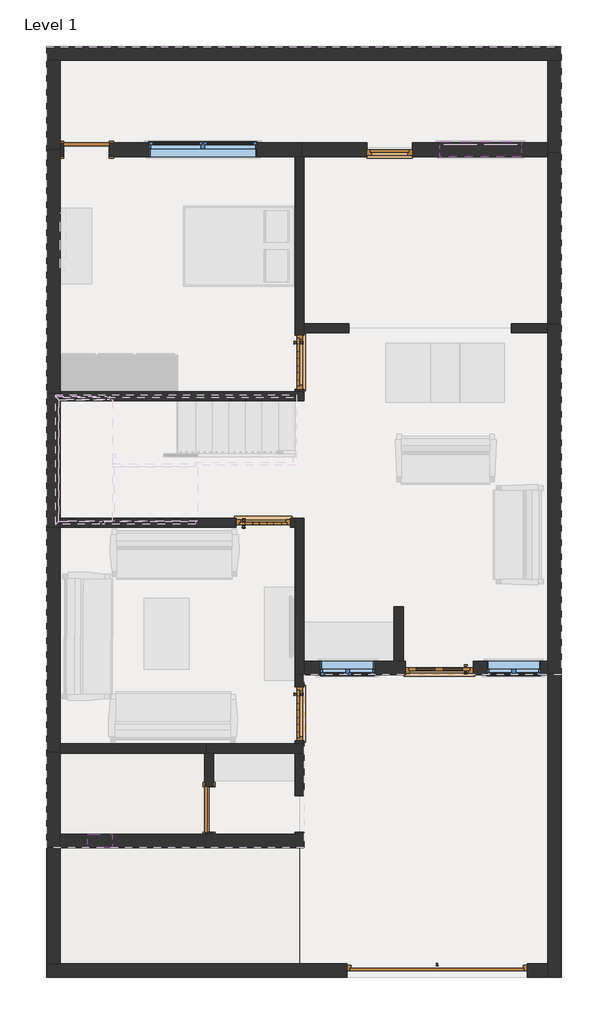
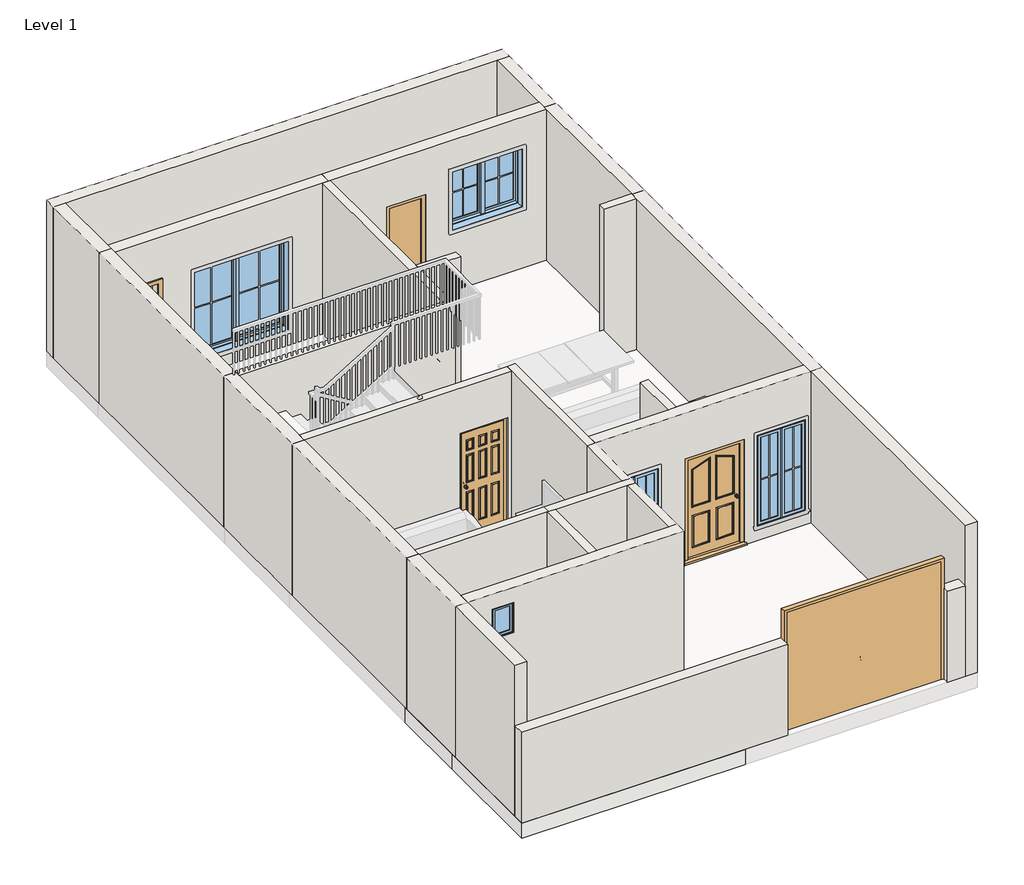
# One storey, part 1 of 3: 28 walls, 8 doors, 5 windows, 2 slabs.
"""IFC4 building model written with IfcOpenShell, lengths in millimetres."""

from ifc_helpers import new_model, si_unit, point, frame, frame_2d, origin, origin_with_axes, place, context, project, spatial, polyline, circle_curve, trimmed, segment, composite_curve, outline, extrude, faceted_brep, transform, mapped, element, save
from components import doors_concept_extsgl_762x2134mm_2_ed5749d6, doors_extsgl_12_1143x2134mm_2_6d3613a0, doors_extsgl_3_914x2134mm_2_3fd9b232, doors_garage_horz_pnl_3048x2438mm_2_abfe55f9, door_e2b13fe9, door_5e1232af, window_aa618e30, window_5590b26e, window_ecc443c5, window_ce442eab

model = new_model("IFC4")

# Units and contexts
model_context = context("Model", 3, world=origin())
ifc_project = project(units=[si_unit("LENGTHUNIT", "METRE", prefix="MILLI")], contexts=[model_context])

# Site, building, storey
site = spatial("IfcSite", under=ifc_project)
building = spatial("IfcBuilding", under=site)
storey = spatial("IfcBuildingStorey", under=building, Name="Level 1", Elevation=0.0)

# Doors
placement = place(None, origin())
doors_concept_extsgl_762x2134mm_2_shape = doors_concept_extsgl_762x2134mm_2_ed5749d6(model_context)
element("IfcDoor", 1, ObjectType="Doors_Concept_ExtSgl : 762x2134mm 2", at=placement, inside=storey, context=model_context, shape_type="MappedRepresentation", body=[
    mapped(doors_concept_extsgl_762x2134mm_2_shape, transform((214.6994028, 7031.3870892, 0.0), x_axis=(-1.0, 0.0, 0.0), y_axis=(0.0, -1.0, 0.0), z_axis=(0.0, 0.0, 1.0))),
])
doors_extsgl_12_1143x2134mm_2_shape = doors_extsgl_12_1143x2134mm_2_6d3613a0(model_context)
element("IfcDoor", 2, ObjectType="Doors_ExtSgl_12 : 1143x2134mm 2", at=placement, inside=storey, context=model_context, shape_type="MappedRepresentation", body=[
    mapped(doors_extsgl_12_1143x2134mm_2_shape, transform((1052.8994028, -1706.2129108, 0.0), x_axis=(-1.0, 0.0, 0.0), y_axis=(0.0, -1.0, 0.0), z_axis=(0.0, 0.0, 1.0))),
])
doors_extsgl_3_914x2134mm_2_shape = doors_extsgl_3_914x2134mm_2_3fd9b232(model_context)
element("IfcDoor", 3, ObjectType="Doors_ExtSgl_3 : 914x2134mm 2", at=placement, inside=storey, context=model_context, shape_type="MappedRepresentation", body=[
    mapped(doors_extsgl_3_914x2134mm_2_shape, transform((-1918.9339305, 744.8870892, 0.0), x_axis=(1.0, 0.0, 0.0), y_axis=(0.0, 1.0, 0.0), z_axis=(0.0, 0.0, 1.0))),
])
element("IfcDoor", 4, ObjectType="Doors_ExtSgl_3 : 914x2134mm 2", at=placement, inside=storey, context=model_context, shape_type="MappedRepresentation", body=[
    mapped(doors_extsgl_3_914x2134mm_2_shape, transform((-1309.3005972, -2480.8795775, 0.0), x_axis=(0.0, -1.0, 0.0), y_axis=(1.0, 0.0, 0.0), z_axis=(0.0, 0.0, 1.0))),
])
element("IfcDoor", 5, ObjectType="Doors_ExtSgl_3 : 914x2134mm 2", at=placement, inside=storey, context=model_context, shape_type="MappedRepresentation", body=[
    mapped(doors_extsgl_3_914x2134mm_2_shape, transform((-1309.3005972, 3450.0204225, 0.0), x_axis=(0.0, -1.0, 0.0), y_axis=(1.0, 0.0, 0.0), z_axis=(0.0, 0.0, 1.0))),
])
doors_garage_horz_pnl_3048x2438mm_2_shape = doors_garage_horz_pnl_3048x2438mm_2_abfe55f9(model_context)
element("IfcDoor", 6, ObjectType="Doors_Garage_Horz_Pnl : 3048x2438mm 2", at=placement, inside=storey, context=model_context, shape_type="MappedRepresentation", body=[
    mapped(doors_garage_horz_pnl_3048x2438mm_2_shape, transform((626.2994028, -6811.6129108, 0.0), x_axis=(1.0, 0.0, 0.0), y_axis=(0.0, 1.0, 0.0), z_axis=(0.0, 0.0, 1.0))),
])
door_shape = door_e2b13fe9(model_context)
element("IfcDoor", 7, ObjectType="Single-Flush : 30\" x 80\" 2", at=placement, inside=storey, context=model_context, shape_type="MappedRepresentation", body=[
    mapped(door_shape, transform((-2833.3005972, -4093.8129108, 0.0), x_axis=(0.0, -1.0, 0.0), y_axis=(1.0, 0.0, 0.0), z_axis=(0.0, 0.0, 1.0))),
])
door_2_shape = door_5e1232af(model_context)
element("IfcDoor", 8, ObjectType="Single-Flush : 30\" x 80\" 2", at=placement, inside=storey, context=model_context, shape_type="MappedRepresentation", body=[
    mapped(door_2_shape, transform((-4903.4005972, 7031.3870892, 0.0), x_axis=(-1.0, 0.0, 0.0), y_axis=(0.0, -1.0, 0.0), z_axis=(0.0, 0.0, 1.0))),
])

# Slabs
element("IfcSlab", 9, ObjectType="Generic - 12\"", at=placement, inside=storey, context=model_context, shape_type="SweptSolid", body=[
    extrude(outline(polyline([(-2833.3005972, -3065.1129108), (-2833.3005972, -4627.2129108), (-5576.5005972, -4627.2129108), (-5576.5005972, -3065.1129108), (-2833.3005972, -3065.1129108)])), frame((0.0, 0.0, -304.8), z_axis=(0.0, 0.0, 1.0), x_axis=(1.0, 0.0, 0.0)), (0.0, 0.0, 1.0), 304.8),
])
element("IfcSlab", 10, ObjectType="Generic - 12\"", at=placement, inside=storey, context=model_context, shape_type="SweptSolid", body=[
    extrude(outline(polyline([(-1309.3005972, -4627.2129108), (-1309.3005972, -6925.9129108), (-5576.5005972, -6925.9129108), (-5576.5005972, -4627.2129108), (-1309.3005972, -4627.2129108)])), frame((0.0, 0.0, -304.8), z_axis=(0.0, 0.0, 1.0), x_axis=(1.0, 0.0, 0.0)), (0.0, 0.0, 1.0), 304.8),
])

# Walls
element("IfcWall", 11, ObjectType="Generic - 8\" 9\"", at=placement, inside=storey, context=model_context, shape_type="Brep", body=[
    faceted_brep([(-5576.5005972, 8542.6870892, 0.0), (-5347.9005972, 8542.6870892, 0.0), (2881.6994028, 8542.6870892, 0.0), (3110.2994028, 8542.6870892, 0.0), (3110.2994028, 8542.6870892, 3048.0), (2881.6994028, 8542.6870892, 3048.0), (-5347.9005972, 8542.6870892, 3048.0), (-5576.5005972, 8542.6870892, 3048.0), (-5576.5005972, 8771.2870892, 0.0), (-5576.5005972, 8771.2870892, 3048.0), (3110.2994028, 8771.2870892, 3048.0), (3110.2994028, 8771.2870892, 0.0)], [[[0, 1, 2, 3, 4, 5, 6, 7]], [[8, 9, 10, 11]], [[3, 2, 1, 0, 8, 11]], [[7, 6, 5, 4, 10, 9]], [[4, 3, 11, 10]], [[0, 7, 9, 8]]]),
])
element("IfcWall", 12, ObjectType="Generic - 8\" 9\"", at=placement, inside=storey, context=model_context, shape_type="Brep", body=[
    faceted_brep([(2881.6994028, 8542.6870892, 0.0), (2881.6994028, 7145.6870892, 0.0), (2881.6994028, 6980.5870892, 0.0), (2881.6994028, 6980.5870892, 3048.0), (2881.6994028, 7145.6870892, 3048.0), (2881.6994028, 8542.6870892, 3048.0), (3110.2994028, 8542.6870892, 0.0), (3110.2994028, 8542.6870892, 3048.0), (3110.2994028, 6980.5870892, 3048.0), (3110.2994028, 6980.5870892, 0.0)], [[[0, 1, 2, 3, 4, 5]], [[6, 7, 8, 9]], [[2, 1, 0, 6, 9]], [[3, 2, 9, 8]], [[5, 4, 3, 8, 7]], [[0, 5, 7, 6]]]),
])
element("IfcWall", 13, ObjectType="Generic - 8\" 9\"", at=placement, inside=storey, context=model_context, shape_type="Brep", body=[
    faceted_brep([(2881.6994028, -6697.3129108, 1828.8), (2881.6994028, -6697.3129108, 0.0), (2538.7994028, -6697.3129108, 0.0), (2538.7994028, -6697.3129108, 1828.8), (2881.6994028, -6925.9129108, 0.0), (2881.6994028, -6925.9129108, 1828.8), (2538.7994028, -6925.9129108, 1828.8), (2538.7994028, -6925.9129108, 0.0)], [[[0, 1, 2, 3]], [[4, 5, 6, 7]], [[1, 4, 7, 2]], [[5, 0, 3, 6]], [[1, 0, 5, 4]], [[3, 2, 7, 6]]]),
    faceted_brep([(-5576.5005972, -6697.3129108, 0.0), (-5576.5005972, -6697.3129108, 1828.8), (-509.2005972, -6697.3129108, 1828.8), (-509.2005972, -6697.3129108, 0.0), (-5347.9005972, -6697.3129108, 0.0), (-5576.5005972, -6925.9129108, 1828.8), (-5576.5005972, -6925.9129108, 0.0), (-509.2005972, -6925.9129108, 0.0), (-509.2005972, -6925.9129108, 1828.8)], [[[0, 1, 2, 3, 4]], [[5, 6, 7, 8]], [[6, 0, 4, 3, 7]], [[1, 5, 8, 2]], [[1, 0, 6, 5]], [[3, 2, 8, 7]]]),
])
element("IfcWall", 14, ObjectType="Generic - 8\" 9\"", at=placement, inside=storey, context=model_context, shape_type="Brep", body=[
    faceted_brep([(-5576.5005972, 8542.6870892, 0.0), (-5576.5005972, 7031.3870892, 0.0), (-5576.5005972, 7031.3870892, 3048.0), (-5576.5005972, 8542.6870892, 3048.0), (-5347.9005972, 8542.6870892, 0.0), (-5347.9005972, 8542.6870892, 3048.0), (-5347.9005972, 7145.6870892, 3048.0), (-5347.9005972, 7031.3870892, 3048.0), (-5347.9005972, 7031.3870892, 0.0), (-5347.9005972, 7145.6870892, 0.0)], [[[0, 1, 2, 3]], [[4, 5, 6, 7, 8, 9]], [[1, 0, 4, 9, 8]], [[2, 1, 8, 7]], [[3, 2, 7, 6, 5]], [[0, 3, 5, 4]]]),
])
element("IfcWall", 15, ObjectType="Generic - 8\" 9\"", at=placement, inside=storey, context=model_context, shape_type="Brep", body=[
    faceted_brep([(-5347.9005972, -4741.5129108, 0.0), (-1233.1005972, -4741.5129108, 0.0), (-1233.1005972, -4741.5129108, 3048.0), (-5347.9005972, -4741.5129108, 3048.0), (-4878.0005972, -4741.5129108, 2743.2), (-4471.6005972, -4741.5129108, 2743.2), (-4471.6005972, -4741.5129108, 2133.6), (-4878.0005972, -4741.5129108, 2133.6), (-5347.9005972, -4512.9129108, 0.0), (-5347.9005972, -4512.9129108, 3048.0), (-2909.5005972, -4512.9129108, 3048.0), (-2757.1005972, -4512.9129108, 3048.0), (-1385.5005972, -4512.9129108, 3048.0), (-1233.1005972, -4512.9129108, 3048.0), (-1233.1005972, -4512.9129108, 0.0), (-1385.5005972, -4512.9129108, 0.0), (-2757.1005972, -4512.9129108, 0.0), (-2909.5005972, -4512.9129108, 0.0), (-4878.0005972, -4512.9129108, 2743.2), (-4878.0005972, -4512.9129108, 2133.6), (-4471.6005972, -4512.9129108, 2133.6), (-4471.6005972, -4512.9129108, 2743.2)], [[[0, 1, 2, 3], [4, 5, 6, 7]], [[8, 9, 10, 11, 12, 13, 14, 15, 16, 17], [18, 19, 20, 21]], [[1, 0, 8, 17, 16, 15, 14]], [[3, 2, 13, 12, 11, 10, 9]], [[0, 3, 9, 8]], [[2, 1, 14, 13]], [[19, 18, 4, 7]], [[20, 19, 7, 6]], [[21, 20, 6, 5]], [[18, 21, 5, 4]]]),
])
element("IfcWall", 16, ObjectType="Generic - 8\" 9\"", at=placement, inside=storey, context=model_context, shape_type="Brep", body=[
    faceted_brep([(481.3994028, -1591.9129108, 2133.6), (481.3994028, -1591.9129108, 0.0), (443.2994028, -1591.9129108, 0.0), (290.8994028, -1591.9129108, 0.0), (-1233.1005972, -1591.9129108, 0.0), (-1233.1005972, -1591.9129108, 3048.0), (290.8994028, -1591.9129108, 3048.0), (443.2994028, -1591.9129108, 3048.0), (2881.6994028, -1591.9129108, 3048.0), (2881.6994028, -1591.9129108, 0.0), (1624.3994028, -1591.9129108, 0.0), (1624.3994028, -1591.9129108, 2133.6), (-953.7005972, -1591.9129108, 2133.6), (-953.7005972, -1591.9129108, 304.8), (-39.3005972, -1591.9129108, 304.8), (-39.3005972, -1591.9129108, 2133.6), (1852.9994028, -1591.9129108, 2133.6), (1852.9994028, -1591.9129108, 304.8), (2767.3994028, -1591.9129108, 304.8), (2767.3994028, -1591.9129108, 2133.6), (-1233.1005972, -1820.5129108, 0.0), (481.3994028, -1820.5129108, 0.0), (481.3994028, -1820.5129108, 2133.6), (1624.3994028, -1820.5129108, 2133.6), (1624.3994028, -1820.5129108, 0.0), (2881.6994028, -1820.5129108, 0.0), (2881.6994028, -1820.5129108, 3048.0), (-1233.1005972, -1820.5129108, 3048.0), (-953.7005972, -1820.5129108, 2133.6), (-39.3005972, -1820.5129108, 2133.6), (-39.3005972, -1820.5129108, 304.8), (-953.7005972, -1820.5129108, 304.8), (1852.9994028, -1820.5129108, 2133.6), (2767.3994028, -1820.5129108, 2133.6), (2767.3994028, -1820.5129108, 304.8), (1852.9994028, -1820.5129108, 304.8), (2881.6994028, -1807.8129108, 0.0), (2881.6994028, -1807.8129108, 3048.0)], [[[0, 1, 2, 3, 4, 5, 6, 7, 8, 9, 10, 11], [12, 13, 14, 15], [16, 17, 18, 19]], [[20, 21, 22, 23, 24, 25, 26, 27], [28, 29, 30, 31], [32, 33, 34, 35]], [[10, 9, 36, 25, 24]], [[4, 3, 2, 1, 21, 20]], [[8, 7, 6, 5, 27, 26, 37]], [[9, 8, 37, 26, 25, 36]], [[5, 4, 20, 27]], [[24, 23, 11, 10]], [[22, 21, 1, 0]], [[23, 22, 0, 11]], [[13, 12, 28, 31]], [[14, 13, 31, 30]], [[15, 14, 30, 29]], [[12, 15, 29, 28]], [[17, 16, 32, 35]], [[18, 17, 35, 34]], [[19, 18, 34, 33]], [[16, 19, 33, 32]]]),
])
element("IfcWall", 17, ObjectType="Generic - 8\" 9\"", at=placement, inside=storey, context=model_context, shape_type="Brep", body=[
    faceted_brep([(-5347.9005972, 6917.0870892, 0.0), (-5284.4005972, 6917.0870892, 0.0), (-5284.4005972, 6917.0870892, 2133.6), (-4522.4005972, 6917.0870892, 2133.6), (-4522.4005972, 6917.0870892, 0.0), (-1385.5005972, 6917.0870892, 0.0), (-1271.2005972, 6917.0870892, 0.0), (-1271.2005972, 6917.0870892, 3048.0), (-1385.5005972, 6917.0870892, 3048.0), (-5347.9005972, 6917.0870892, 3048.0), (-2020.5005972, 6917.0870892, 2133.6), (-2020.5005972, 6917.0870892, 304.8), (-3849.3005972, 6917.0870892, 304.8), (-3849.3005972, 6917.0870892, 2133.6), (-5284.4005972, 7145.6870892, 2133.6), (-5284.4005972, 7145.6870892, 0.0), (-5347.9005972, 7145.6870892, 0.0), (-5347.9005972, 7145.6870892, 3048.0), (-1271.2005972, 7145.6870892, 3048.0), (-1271.2005972, 7145.6870892, 0.0), (-4522.4005972, 7145.6870892, 0.0), (-4522.4005972, 7145.6870892, 2133.6), (-2020.5005972, 7145.6870892, 2133.6), (-3849.3005972, 7145.6870892, 2133.6), (-3849.3005972, 7145.6870892, 304.8), (-2020.5005972, 7145.6870892, 304.8), (-5347.9005972, 7031.3870892, 0.0), (-5347.9005972, 7031.3870892, 3048.0)], [[[0, 1, 2, 3, 4, 5, 6, 7, 8, 9], [10, 11, 12, 13]], [[14, 15, 16, 17, 18, 19, 20, 21], [22, 23, 24, 25]], [[20, 19, 6, 5, 4]], [[16, 15, 1, 0, 26]], [[7, 6, 19, 18]], [[9, 8, 7, 18, 17, 27]], [[0, 9, 27, 17, 16, 26]], [[2, 1, 15, 14]], [[3, 2, 14, 21]], [[4, 3, 21, 20]], [[11, 10, 22, 25]], [[12, 11, 25, 24]], [[13, 12, 24, 23]], [[10, 13, 23, 22]]]),
])
element("IfcWall", 18, ObjectType="Generic - 8\" 9\"", at=placement, inside=storey, context=model_context, shape_type="Brep", body=[
    faceted_brep([(-5576.5005972, -4741.5129108, 0.0), (-5576.5005972, -6697.3129108, 0.0), (-5576.5005972, -6697.3129108, 1828.8), (-5576.5005972, -6697.3129108, 3048.0), (-5576.5005972, -4741.5129108, 3048.0), (-5347.9005972, -4741.5129108, 0.0), (-5347.9005972, -4741.5129108, 3048.0), (-5347.9005972, -6697.3129108, 3048.0), (-5347.9005972, -6697.3129108, 0.0)], [[[0, 1, 2, 3, 4]], [[5, 6, 7, 8]], [[1, 0, 5, 8]], [[4, 3, 7, 6]], [[3, 2, 1, 8, 7]], [[0, 4, 6, 5]]]),
])
element("IfcWall", 19, ObjectType="Generic - 8\" 9\"", at=placement, inside=storey, context=model_context, shape_type="Brep", body=[
    faceted_brep([(2881.6994028, -1807.8129108, 0.0), (2881.6994028, -1820.5129108, 0.0), (2881.6994028, -6697.3129108, 0.0), (2881.6994028, -6925.9129108, 0.0), (2881.6994028, -6925.9129108, 1828.8), (2881.6994028, -6925.9129108, 3048.0), (2881.6994028, -1820.5129108, 3048.0), (2881.6994028, -1807.8129108, 3048.0), (3110.2994028, -1807.8129108, 0.0), (3110.2994028, -1807.8129108, 3048.0), (3110.2994028, -6925.9129108, 3048.0), (3110.2994028, -6925.9129108, 0.0)], [[[0, 1, 2, 3, 4, 5, 6, 7]], [[8, 9, 10, 11]], [[3, 2, 1, 0, 8, 11]], [[7, 6, 5, 10, 9]], [[0, 7, 9, 8]], [[5, 4, 3, 11, 10]]]),
])
element("IfcWall", 20, ObjectType="Generic - 8\" 9\"", at=placement, inside=storey, context=model_context, shape_type="Brep", body=[
    faceted_brep([(-5576.5005972, -3128.6129108, 0.0), (-5576.5005972, -4741.5129108, 0.0), (-5576.5005972, -4741.5129108, 3048.0), (-5576.5005972, -3128.6129108, 3048.0), (-5347.9005972, -3128.6129108, 0.0), (-5347.9005972, -3128.6129108, 3048.0), (-5347.9005972, -4512.9129108, 3048.0), (-5347.9005972, -4741.5129108, 3048.0), (-5347.9005972, -4741.5129108, 0.0), (-5347.9005972, -4512.9129108, 0.0)], [[[0, 1, 2, 3]], [[4, 5, 6, 7, 8, 9]], [[1, 0, 4, 9, 8]], [[3, 2, 7, 6, 5]], [[0, 3, 5, 4]], [[2, 1, 8, 7]]]),
])
element("IfcWall", 21, ObjectType="Generic - 8\" 9\"", at=placement, inside=storey, context=model_context, shape_type="Brep", body=[
    faceted_brep([(-1271.2005972, 6917.0870892, 0.0), (-166.3005972, 6917.0870892, 0.0), (-166.3005972, 6917.0870892, 2133.6), (595.6994028, 6917.0870892, 2133.6), (595.6994028, 6917.0870892, 0.0), (2881.6994028, 6917.0870892, 0.0), (2881.6994028, 6917.0870892, 3048.0), (-1271.2005972, 6917.0870892, 3048.0), (2437.1994028, 6917.0870892, 2438.4), (2437.1994028, 6917.0870892, 1219.2), (1065.5994028, 6917.0870892, 1219.2), (1065.5994028, 6917.0870892, 2438.4), (-166.3005972, 7145.6870892, 2133.6), (-166.3005972, 7145.6870892, 0.0), (-1271.2005972, 7145.6870892, 0.0), (-1271.2005972, 7145.6870892, 3048.0), (2881.6994028, 7145.6870892, 3048.0), (2881.6994028, 7145.6870892, 0.0), (595.6994028, 7145.6870892, 0.0), (595.6994028, 7145.6870892, 2133.6), (2437.1994028, 7145.6870892, 2438.4), (1065.5994028, 7145.6870892, 2438.4), (1065.5994028, 7145.6870892, 1219.2), (2437.1994028, 7145.6870892, 1219.2), (2881.6994028, 6980.5870892, 0.0), (2881.6994028, 6980.5870892, 3048.0)], [[[0, 1, 2, 3, 4, 5, 6, 7], [8, 9, 10, 11]], [[12, 13, 14, 15, 16, 17, 18, 19], [20, 21, 22, 23]], [[18, 17, 24, 5, 4]], [[14, 13, 1, 0]], [[7, 6, 25, 16, 15]], [[0, 7, 15, 14]], [[6, 5, 24, 17, 16, 25]], [[3, 2, 12, 19]], [[2, 1, 13, 12]], [[4, 3, 19, 18]], [[8, 11, 21, 20]], [[11, 10, 22, 21]], [[10, 9, 23, 22]], [[9, 8, 20, 23]]]),
])
element("IfcWall", 22, ObjectType="Generic - 8\" 9\"", at=placement, inside=storey, context=model_context, shape_type="Brep", body=[
    faceted_brep([(-5576.5005972, 7031.3870892, 0.0), (-5576.5005972, 2916.5870892, 0.0), (-5576.5005972, 2916.5870892, 3048.0), (-5576.5005972, 7031.3870892, 3048.0), (-5347.9005972, 7031.3870892, 0.0), (-5347.9005972, 7031.3870892, 3048.0), (-5347.9005972, 6917.0870892, 3048.0), (-5347.9005972, 2916.5870892, 3048.0), (-5347.9005972, 2916.5870892, 0.0), (-5347.9005972, 6917.0870892, 0.0)], [[[0, 1, 2, 3]], [[4, 5, 6, 7, 8, 9]], [[1, 0, 4, 9, 8]], [[2, 1, 8, 7]], [[3, 2, 7, 6, 5]], [[0, 3, 5, 4]]]),
])
element("IfcWall", 23, ObjectType="Generic - 8\" 9\"", at=placement, inside=storey, context=model_context, shape_type="Brep", body=[
    faceted_brep([(-5576.5005972, 2916.5870892, 0.0), (-5576.5005972, 655.9870892, 0.0), (-5576.5005972, 655.9870892, 3048.0), (-5576.5005972, 2916.5870892, 3048.0), (-5347.9005972, 2916.5870892, 0.0), (-5347.9005972, 2916.5870892, 3048.0), (-5347.9005972, 2802.2870892, 3048.0), (-5347.9005972, 821.0870892, 3048.0), (-5347.9005972, 668.6870892, 3048.0), (-5347.9005972, 655.9870892, 3048.0), (-5347.9005972, 655.9870892, 0.0), (-5347.9005972, 668.6870892, 0.0), (-5347.9005972, 821.0870892, 0.0), (-5347.9005972, 2802.2870892, 0.0)], [[[0, 1, 2, 3]], [[4, 5, 6, 7, 8, 9, 10, 11, 12, 13]], [[1, 0, 4, 13, 12, 11, 10]], [[2, 1, 10, 9]], [[3, 2, 9, 8, 7, 6, 5]], [[0, 3, 5, 4]]]),
])
element("IfcWall", 24, ObjectType="Generic - 8\" 9\"", at=placement, inside=storey, context=model_context, shape_type="Brep", body=[
    faceted_brep([(-5576.5005972, 655.9870892, 0.0), (-5576.5005972, -3128.6129108, 0.0), (-5576.5005972, -3128.6129108, 3048.0), (-5576.5005972, 655.9870892, 3048.0), (-5347.9005972, 655.9870892, 0.0), (-5347.9005972, 655.9870892, 3048.0), (-5347.9005972, -2988.9129108, 3048.0), (-5347.9005972, -3128.6129108, 3048.0), (-5347.9005972, -3128.6129108, 0.0), (-5347.9005972, -2988.9129108, 0.0)], [[[0, 1, 2, 3]], [[4, 5, 6, 7, 8, 9]], [[1, 0, 4, 9, 8]], [[2, 1, 8, 7]], [[3, 2, 7, 6, 5]], [[0, 3, 5, 4]]]),
])
element("IfcWall", 25, ObjectType="Generic - 8\" 9\"", at=placement, inside=storey, context=model_context, shape_type="Brep", body=[
    faceted_brep([(2881.6994028, 4084.9870892, 0.0), (2881.6994028, 3945.2870892, 0.0), (2881.6994028, -1591.9129108, 0.0), (2881.6994028, -1807.8129108, 0.0), (2881.6994028, -1807.8129108, 3048.0), (2881.6994028, -1591.9129108, 3048.0), (2881.6994028, 3945.2870892, 3048.0), (2881.6994028, 4084.9870892, 3048.0), (3110.2994028, 4084.9870892, 0.0), (3110.2994028, 4084.9870892, 3048.0), (3110.2994028, -1807.8129108, 3048.0), (3110.2994028, -1807.8129108, 0.0)], [[[0, 1, 2, 3, 4, 5, 6, 7]], [[8, 9, 10, 11]], [[3, 2, 1, 0, 8, 11]], [[4, 3, 11, 10]], [[7, 6, 5, 4, 10, 9]], [[0, 7, 9, 8]]]),
])
element("IfcWall", 26, ObjectType="Generic - 8\" 9\"", at=placement, inside=storey, context=model_context, shape_type="SweptSolid", body=[
    extrude(outline(polyline([(2881.6994028, 4084.9870892), (2881.6994028, 6980.5870892), (3110.2994028, 6980.5870892), (3110.2994028, 4084.9870892), (2881.6994028, 4084.9870892)])), origin_with_axes(), (0.0, 0.0, 1.0), 3048.0),
])
element("IfcWall", 27, ObjectType="Generic - 8\"6\"", at=placement, inside=storey, context=model_context, shape_type="Brep", body=[
    faceted_brep([(-5347.9005972, -3141.3129108, 0.0), (-2884.1005972, -3141.3129108, 0.0), (-2884.1005972, -3141.3129108, 3048.0), (-5347.9005972, -3141.3129108, 3048.0), (-5347.9005972, -2988.9129108, 0.0), (-5347.9005972, -2988.9129108, 3048.0), (-2884.1005972, -2988.9129108, 3048.0), (-2884.1005972, -2988.9129108, 0.0), (-5347.9005972, -3128.6129108, 0.0), (-5347.9005972, -3128.6129108, 3048.0)], [[[0, 1, 2, 3]], [[4, 5, 6, 7]], [[1, 0, 8, 4, 7]], [[2, 1, 7, 6]], [[3, 2, 6, 5, 9]], [[0, 3, 9, 5, 4, 8]]]),
])
element("IfcWall", 28, ObjectType="Generic - 8\"6\"", at=placement, inside=storey, context=model_context, shape_type="SweptSolid", body=[
    extrude(outline(composite_curve([segment(polyline([(-3141.3129108, 0.0), (-3865.2129108, 0.0), (-3865.2129108, 2133.6)]), True, "CONTINUOUS"), segment(trimmed(circle_curve(frame_2d((-4170.0129108, 2133.6)), 304.8), [point((-3865.2129108, 2133.6))], [point((-4474.8129108, 2133.6))], True, "CARTESIAN"), True, "CONTINUOUS"), segment(polyline([(-4474.8129108, 2133.6), (-4474.8129108, 0.0), (-4512.9129108, 0.0), (-4512.9129108, 3048.0), (-3141.3129108, 3048.0), (-3141.3129108, 0.0)]), True, "CONTINUOUS")], self_intersect=False)), frame((-1385.5005972, 0.0, 0.0), z_axis=(1.0, 0.0, 0.0), x_axis=(0.0, 1.0, 0.0)), (0.0, 0.0, 1.0), 152.4),
])
element("IfcWall", 29, ObjectType="Generic - 8\"6\"", at=placement, inside=storey, context=model_context, shape_type="Brep", body=[
    faceted_brep([(-2909.5005972, -4474.8129108, 2133.6), (-2909.5005972, -4474.8129108, 0.0), (-2909.5005972, -4512.9129108, 0.0), (-2909.5005972, -4512.9129108, 3048.0), (-2909.5005972, -3141.3129108, 3048.0), (-2909.5005972, -3141.3129108, 0.0), (-2909.5005972, -3712.8129108, 0.0), (-2909.5005972, -3712.8129108, 2133.6), (-2757.1005972, -4512.9129108, 0.0), (-2757.1005972, -4474.8129108, 0.0), (-2757.1005972, -4474.8129108, 2133.6), (-2757.1005972, -3712.8129108, 2133.6), (-2757.1005972, -3712.8129108, 0.0), (-2757.1005972, -3141.3129108, 0.0), (-2757.1005972, -3141.3129108, 3048.0), (-2757.1005972, -4512.9129108, 3048.0), (-2884.1005972, -3141.3129108, 0.0), (-2884.1005972, -3141.3129108, 3048.0)], [[[0, 1, 2, 3, 4, 5, 6, 7]], [[8, 9, 10, 11, 12, 13, 14, 15]], [[6, 5, 16, 13, 12]], [[2, 1, 9, 8]], [[4, 3, 15, 14, 17]], [[3, 2, 8, 15]], [[5, 4, 17, 14, 13, 16]], [[10, 9, 1, 0]], [[11, 10, 0, 7]], [[12, 11, 7, 6]]]),
])
element("IfcWall", 30, ObjectType="Generic - 8\"6\"", at=placement, inside=storey, context=model_context, shape_type="SweptSolid", body=[
    extrude(outline(polyline([(-2938.1129108, 2133.6), (-2938.1129108, 0.0), (-2988.9129108, 0.0), (-2988.9129108, 3048.0), (-1820.5129108, 3048.0), (-1820.5129108, 0.0), (-2023.7129108, 0.0), (-2023.7129108, 2133.6), (-2938.1129108, 2133.6)])), frame((-1385.5005972, 0.0, 0.0), z_axis=(1.0, 0.0, 0.0), x_axis=(0.0, 1.0, 0.0)), (0.0, 0.0, 1.0), 152.4),
])
element("IfcWall", 31, ObjectType="Generic - 8\"6\"", at=placement, inside=storey, context=model_context, shape_type="SweptSolid", body=[
    extrude(outline(polyline([(2133.6, -1461.7005972), (0.0, -1461.7005972), (0.0, -1385.5005972), (3048.0, -1385.5005972), (3048.0, -5347.9005972), (0.0, -5347.9005972), (0.0, -2376.1005972), (2133.6, -2376.1005972), (2133.6, -1461.7005972)])), frame((0.0, 668.6870892, 0.0), z_axis=(0.0, 1.0, 0.0), x_axis=(0.0, 0.0, 1.0)), (0.0, 0.0, 1.0), 152.4),
])
element("IfcWall", 32, ObjectType="Generic - 8\"6\"", at=placement, inside=storey, context=model_context, shape_type="Brep", body=[
    faceted_brep([(-5347.9005972, 2802.2870892, 0.0), (-1233.1005972, 2802.2870892, 0.0), (-1233.1005972, 2802.2870892, 3048.0), (-5347.9005972, 2802.2870892, 3048.0), (-5347.9005972, 2954.6870892, 0.0), (-5347.9005972, 2954.6870892, 3048.0), (-1385.5005972, 2954.6870892, 3048.0), (-1233.1005972, 2954.6870892, 3048.0), (-1233.1005972, 2954.6870892, 0.0), (-1385.5005972, 2954.6870892, 0.0), (-5347.9005972, 2916.5870892, 0.0), (-5347.9005972, 2916.5870892, 3048.0)], [[[0, 1, 2, 3]], [[4, 5, 6, 7, 8, 9]], [[1, 0, 10, 4, 9, 8]], [[3, 2, 7, 6, 5, 11]], [[0, 3, 11, 5, 4, 10]], [[2, 1, 8, 7]]]),
])
element("IfcWall", 33, ObjectType="Generic - 8\"6\"", at=placement, inside=storey, context=model_context, shape_type="Brep", body=[
    faceted_brep([(-1233.1005972, 2954.6870892, 0.0), (-1233.1005972, 2992.7870892, 0.0), (-1233.1005972, 2992.7870892, 2133.6), (-1233.1005972, 3907.1870892, 2133.6), (-1233.1005972, 3907.1870892, 0.0), (-1233.1005972, 3945.2870892, 0.0), (-1233.1005972, 4097.6870892, 0.0), (-1233.1005972, 6917.0870892, 0.0), (-1233.1005972, 6917.0870892, 3048.0), (-1233.1005972, 4097.6870892, 3048.0), (-1233.1005972, 3945.2870892, 3048.0), (-1233.1005972, 2954.6870892, 3048.0), (-1385.5005972, 2992.7870892, 2133.6), (-1385.5005972, 2992.7870892, 0.0), (-1385.5005972, 2954.6870892, 0.0), (-1385.5005972, 2954.6870892, 3048.0), (-1385.5005972, 6917.0870892, 3048.0), (-1385.5005972, 6917.0870892, 0.0), (-1385.5005972, 3907.1870892, 0.0), (-1385.5005972, 3907.1870892, 2133.6), (-1271.2005972, 6917.0870892, 0.0), (-1271.2005972, 6917.0870892, 3048.0)], [[[0, 1, 2, 3, 4, 5, 6, 7, 8, 9, 10, 11]], [[12, 13, 14, 15, 16, 17, 18, 19]], [[18, 17, 20, 7, 6, 5, 4]], [[14, 13, 1, 0]], [[11, 10, 9, 8, 21, 16, 15]], [[0, 11, 15, 14]], [[8, 7, 20, 17, 16, 21]], [[4, 3, 19, 18]], [[2, 1, 13, 12]], [[3, 2, 12, 19]]]),
])
element("IfcWall", 34, ObjectType="Generic - 8\"6\"", at=placement, inside=storey, context=model_context, shape_type="SweptSolid", body=[
    extrude(outline(polyline([(-468.1553791, 3945.2870892), (-1233.1005972, 3945.2870892), (-1233.1005972, 4097.6870892), (-468.1553791, 4097.6870892), (-468.1553791, 3945.2870892)])), origin_with_axes(), (0.0, 0.0, 1.0), 3048.0),
])
element("IfcWall", 35, ObjectType="Generic - 8\"6\"", at=placement, inside=storey, context=model_context, shape_type="Brep", body=[
    faceted_brep([(2881.6994028, 4097.6870892, 0.0), (2272.0994028, 4097.6870892, 0.0), (2272.0994028, 4097.6870892, 3048.0), (2881.6994028, 4097.6870892, 3048.0), (2881.6994028, 3945.2870892, 0.0), (2881.6994028, 3945.2870892, 3048.0), (2272.0994028, 3945.2870892, 3048.0), (2272.0994028, 3945.2870892, 0.0), (2881.6994028, 4084.9870892, 0.0), (2881.6994028, 4084.9870892, 3048.0)], [[[0, 1, 2, 3]], [[4, 5, 6, 7]], [[1, 0, 8, 4, 7]], [[2, 1, 7, 6]], [[3, 2, 6, 5, 9]], [[0, 3, 9, 5, 4, 8]]]),
])
element("IfcWall", 36, ObjectType="Generic - 8\"6\"", at=placement, inside=storey, context=model_context, shape_type="SweptSolid", body=[
    extrude(outline(polyline([(443.2994028, -677.5129108), (443.2994028, -1591.9129108), (290.8994028, -1591.9129108), (290.8994028, -677.5129108), (443.2994028, -677.5129108)])), origin_with_axes(), (0.0, 0.0, 1.0), 3048.0),
])
element("IfcWall", 37, ObjectType="Generic - 8\"6\"", at=placement, inside=storey, context=model_context, shape_type="Brep", body=[
    faceted_brep([(-1233.1005972, -1820.5129108, 0.0), (-1233.1005972, -1591.9129108, 0.0), (-1233.1005972, 821.0870892, 0.0), (-1233.1005972, 821.0870892, 3048.0), (-1233.1005972, -1591.9129108, 3048.0), (-1233.1005972, -1820.5129108, 3048.0), (-1385.5005972, -1820.5129108, 0.0), (-1385.5005972, -1820.5129108, 3048.0), (-1385.5005972, 668.6870892, 3048.0), (-1385.5005972, 821.0870892, 3048.0), (-1385.5005972, 821.0870892, 0.0), (-1385.5005972, 668.6870892, 0.0)], [[[0, 1, 2, 3, 4, 5]], [[6, 7, 8, 9, 10, 11]], [[2, 1, 0, 6, 11, 10]], [[5, 4, 3, 9, 8, 7]], [[0, 5, 7, 6]], [[3, 2, 10, 9]]]),
])
element("IfcWall", 38, ObjectType="Generic - 8\"6\"", at=placement, inside=storey, context=model_context, shape_type="Brep", body=[
    faceted_brep([(-2884.1005972, -3141.3129108, 0.0), (-2757.1005972, -3141.3129108, 0.0), (-1385.5005972, -3141.3129108, 0.0), (-1233.1005972, -3141.3129108, 0.0), (-1233.1005972, -3141.3129108, 3048.0), (-1385.5005972, -3141.3129108, 3048.0), (-2757.1005972, -3141.3129108, 3048.0), (-2884.1005972, -3141.3129108, 3048.0), (-2884.1005972, -2988.9129108, 0.0), (-2884.1005972, -2988.9129108, 3048.0), (-1385.5005972, -2988.9129108, 3048.0), (-1233.1005972, -2988.9129108, 3048.0), (-1233.1005972, -2988.9129108, 0.0), (-1385.5005972, -2988.9129108, 0.0)], [[[0, 1, 2, 3, 4, 5, 6, 7]], [[8, 9, 10, 11, 12, 13]], [[3, 2, 1, 0, 8, 13, 12]], [[7, 6, 5, 4, 11, 10, 9]], [[0, 7, 9, 8]], [[4, 3, 12, 11]]]),
])

# Windows
window_shape = window_aa618e30(model_context)
element("IfcWindow", 39, ObjectType="Fixed : 16\" x 24\" 2", at=placement, inside=storey, context=model_context, shape_type="MappedRepresentation", body=[
    mapped(window_shape, transform((-4712.9005972, -4627.2129108, 1219.2), x_axis=(-1.0, 0.0, 0.0), y_axis=(0.0, -1.0, 0.0), z_axis=(0.0, 0.0, 1.0))),
])
window_2_shape = window_5590b26e(model_context)
element("IfcWindow", 40, ObjectType="Window-Casement-Double : 36\" x 72\"", at=placement, inside=storey, context=model_context, shape_type="MappedRepresentation", body=[
    mapped(window_2_shape, transform((-496.5005972, -1706.2129108, -609.6), x_axis=(-1.0, 0.0, 0.0), y_axis=(0.0, -1.0, 0.0), z_axis=(0.0, 0.0, 1.0))),
])
element("IfcWindow", 41, ObjectType="Window-Casement-Double : 36\" x 72\"", at=placement, inside=storey, context=model_context, shape_type="MappedRepresentation", body=[
    mapped(window_2_shape, transform((2310.1994028, -1706.2129108, -609.6), x_axis=(-1.0, 0.0, 0.0), y_axis=(0.0, -1.0, 0.0), z_axis=(0.0, 0.0, 1.0))),
])
window_3_shape = window_ecc443c5(model_context)
element("IfcWindow", 42, ObjectType="Window-Casement-Double : 54\" x 48\"", at=placement, inside=storey, context=model_context, shape_type="MappedRepresentation", body=[
    mapped(window_3_shape, transform((1751.3994028, 7031.3870892, 304.8), x_axis=(1.0, 0.0, 0.0), y_axis=(0.0, 1.0, 0.0), z_axis=(0.0, 0.0, 1.0))),
])
window_4_shape = window_ce442eab(model_context)
element("IfcWindow", 43, ObjectType="Window-Casement-Double : 72\" x 72\"", at=placement, inside=storey, context=model_context, shape_type="MappedRepresentation", body=[
    mapped(window_4_shape, transform((-2934.9005972, 7031.3870892, -609.6), x_axis=(1.0, 0.0, 0.0), y_axis=(0.0, 1.0, 0.0), z_axis=(0.0, 0.0, 1.0))),
])

save(model, "model.ifc")

# Revit data of these elements
# Type "Doors_Concept_ExtSgl : 762x2134mm 2"
#   Type Mark = "17"
#   Type Comments = "External Single"
#   Operation = "SingleSwingRight"
#   Construction Type Id = "SGL"
#   Keynote = "L10"
#   Analytic Construction = "Large single-glazed windows"
#   Visual Light Transmittance = 0.9
#   Thickness = 0' - 1.73228"
#   Solar Heat Gain Coefficient = 0.86
#   Rough Width = 2' - 6"
#   Rough Height = 7' - 0"
#   Heat Transfer Coefficient (U) = 0.979472 BTU/(h·ft²·°F)
#   FrameWidth = 0' - 1.65354"
#   FrameOffset - External = 0' - 0.98425"
#   Height = 7' - 0"
#   Width = 2' - 6"
#   Define Thermal Properties by = 1
#   Function = 1
#   Material Door = Concept
#   Material Frame = Concept
#   Wall Closure = (empty or 0)
#   Assembly Code = ""
# Type "Doors_ExtSgl_12 : 1143x2134mm 2"
#   Type Mark = "10"
#   Type Comments = "External Single"
#   Operation = "SingleSwingRight"
#   Construction Type Id = "SGL"
#   Keynote = "L20"
#   Analytic Construction = "Large single-glazed windows"
#   Wrap Layers (Int) from Ext = 0' - 6.98819"
#   Wrap Layers (Ext) from Ext = 0' - 4.03543"
#   Visual Light Transmittance = 0.9
#   Thickness = 0' - 1.73228"
#   Stile Top of Lock rail = 3' - 3.37008"
#   Stile Top Rail = 0' - 5.90551"
#   Stile Shutting = 0' - 4.92126"
#   Stile Muntin Rail = 0' - 4.92126"
#   Stile Lock Rail = 0' - 6.88976"
#   Stile Hanging = 0' - 4.92126"
#   Stile Bottom Rail = 0' - 6.88976"
#   Solar Heat Gain Coefficient = 0.86
#   Rough Width = 3' - 9"
#   Rough Height = 7' - 0"
#   O/A Frame Width = 0' - 2.51969"
#   Heat Transfer Coefficient (U) = 0.979472 BTU/(h·ft²·°F)
#   Handle Z Distance = 3' - 3.37008"
#   Glazing Thickness = 0' - 0.94488"
#   FrameWidth = 0' - 1.65354"
#   FrameOffset - External = 0' - 0.98425"
#   FrameDepth = 0' - 3.50394"
#   Door Panel Width = 3' - 4.94488"
#   Door Panel Thickness = 0' - 1.73228"
#   Door Panel Height = 6' - 7.66929"
#   Cill Thickness = 0' - 2.14567"
#   Cill Projection = 0' - 1.1811"
#   Handle X Distance = 0' - 2.95276"
#   Height = 7' - 0"
#   Structural Tolerance = 0' - 0.25591"
#   Tolerance = 0' - 0.11811"
#   Undercut = 0' - 0.15748"
#   Width = 3' - 9"
#   Cill Extension = 0' - 0.98425"
#   Cavity Closer Width = 0' - 1.9685"
#   Cavity Closer Offset from Ext = 0' - 4.03543"
#   Cavity Closer Depth = 0' - 3.34646"
#   Vis - Ironmongery = yes
#   Vis - Cavity Closers = yes
#   Define Thermal Properties by = 1
#   Function = 1
#   Material Glass = Door - Glazing
#   Material Door = Door - Panel
#   Material Frame = Door - Frame/Mullion
#   Material Ironmongery = Door - Handle
#   Wall Closure = (empty or 0)
# Type "Doors_ExtSgl_3 : 914x2134mm 2"
#   Type Mark = "13"
#   Type Comments = "External Single"
#   Operation = "SingleSwingRight"
#   Construction Type Id = "MDOOR"
#   Keynote = "L20"
#   Analytic Construction = "Metal"
#   Wrap Layers (Int) from Ext = 0' - 6.98819"
#   Wrap Layers (Ext) from Ext = 0' - 4.03543"
#   Thickness = 0' - 1.73228"
#   Stile Top of Lock rail = 3' - 3.37008"
#   Stile Top of Frieze Rail = 5' - 4.96063"
#   Stile Top Rail = 0' - 5.90551"
#   Stile Shutting = 0' - 3.54331"
#   Stile Muntin Rail = 0' - 3.54331"
#   Stile Lock Rail = 0' - 6.88976"
#   Stile Intermediate/Frieze = 0' - 3.14961"
#   Stile Hanging = 0' - 3.54331"
#   Stile Bottom Rail = 0' - 6.88976"
#   Rough Width = 3' - 0"
#   Rough Height = 7' - 0"
#   O/A Frame Width = 0' - 2.51969"
#   Heat Transfer Coefficient (U) = 0.651978 BTU/(h·ft²·°F)
#   Handle Z Distance = 3' - 3.37008"
#   Glazing Thickness = 0' - 0.94488"
#   FrameWidth = 0' - 1.65354"
#   FrameOffset - External = 0' - 0.98425"
#   FrameDepth = 0' - 3.50394"
#   Door Panel Width = 2' - 7.94488"
#   Door Panel Thickness = 0' - 1.73228"
#   Door Panel Height = 6' - 7.66929"
#   DONT CHANGE - Panel Width = 0' - 5.92388"
#   Cill Thickness = 0' - 2.14567"
#   Cill Projection = 0' - 1.1811"
#   Handle X Distance = 0' - 2.95276"
#   Height = 7' - 0"
#   Structural Tolerance = 0' - 0.25591"
#   Tolerance = 0' - 0.11811"
#   Undercut = 0' - 0.15748"
#   Width = 3' - 0"
#   Cill Extension = 0' - 0.98425"
#   Cavity Closer Width = 0' - 1.9685"
#   Cavity Closer Offset from Ext = 0' - 4.03543"
#   Cavity Closer Depth = 0' - 3.34646"
#   Vis - Ironmongery = yes
#   Vis - Cavity Closers = yes
#   Define Thermal Properties by = 1
#   Function = 1
#   Material Door = Door - Panel
#   Material Frame = Door - Frame/Mullion
#   Material Ironmongery = Door - Handle
#   Visual Light Transmittance = 0
#   Solar Heat Gain Coefficient = 0
#   Wall Closure = (empty or 0)
# Type "Doors_Garage_Horz_Pnl : 3048x2438mm 2"
#   Type Mark = "20"
#   Type Comments = "External Garage"
#   Operation = "RollingUp"
#   Construction Type Id = "MDOOR"
#   Keynote = "L20"
#   Analytic Construction = "Metal"
#   Wrap Layers (Ext) from Ext = 0' - 4.03543"
#   Wrap Layers (Int) from Ext = 0' - 6.98819"
#   Thickness = 0' - 1.73228"
#   Rough Width = 10' - 0"
#   Rough Height = 8' - 0"
#   O/A Frame Width = 0' - 2.51969"
#   Heat Transfer Coefficient (U) = 0.651978 BTU/(h·ft²·°F)
#   Handle Z Distance = 2' - 11.43307"
#   FrameWidth = 0' - 1.65354"
#   FrameOffset - External = 0' - 0.98425"
#   FrameDepth = 0' - 3.50394"
#   Door Panel Thickness = 0' - 1.73228"
#   Height = 8' - 0"
#   Structural Tolerance = 0' - 0.25591"
#   Tolerance = 0' - 0.11811"
#   Undercut = 0' - 0.3937"
#   Width = 10' - 0"
#   Cavity Closer Width = 0' - 1.9685"
#   Cavity Closer Offset from Ext = 0' - 4.03543"
#   Cavity Closer Depth = 0' - 2.95276"
#   Vis - Ironmongery = yes
#   Vis - Cavity Closers = yes
#   Define Thermal Properties by = 1
#   Function = 1
#   Material Door = Door - Panel
#   Material Frame = Door - Frame/Mullion
#   Material Ironmongery = Door - Handle
#   Visual Light Transmittance = 0
#   Solar Heat Gain Coefficient = 0
#   Wall Closure = (empty or 0)
# Type "Single-Flush : 30\" x 80\" 2"
#   Type Mark = "14"
#   Construction Type Id = "MDOOR"
#   Assembly Code = "C1020"
#   Analytic Construction = "Metal"
#   Thickness = 0' - 2"
#   Heat Transfer Coefficient (U) = 0.651978 BTU/(h·ft²·°F)
#   Height = 7' - 0"
#   Trim Projection Ext = 0' - 1"
#   Trim Projection Int = 0' - 1"
#   Trim Width = 0' - 3"
#   Width = 2' - 6"
#   Define Thermal Properties by = 1
#   Door Material = Door - Panel
#   Frame Material = Door - Frame
#   Visual Light Transmittance = 0
#   Solar Heat Gain Coefficient = 0
#   Function = (empty or 0)
#   Wall Closure = (empty or 0)
# Type "Generic - 12\""
#   Assembly Code = "B1010"
#   Function = 0
#   Layers, outside or top first: 1' - 0" no material (function 1)
# Type "Generic - 8\" 9\""
#   Assembly Code = "B2010"
#   Layers, outside or top first: 0' - 9" no material (function 1)
# Type "Generic - 8\"6\""
#   Assembly Code = "B2010"
#   Layers, outside or top first: 0' - 6" no material (function 1)
# Type "Fixed : 16\" x 24\" 2"
#   Type Mark = "21"
#   Construction Type Id = "GSP4R"
#   Assembly Code = "B2020100"
#   Analytic Construction = "1/8 in Pilkington single glazing"
#   Visual Light Transmittance = 0.9
#   Solar Heat Gain Coefficient = 0.78
#   Heat Transfer Coefficient (U) = 0.6496 BTU/(h·ft²·°F)
#   Height = 2' - 0"
#   Default Sill Height = 3' - 0"
#   Width = 1' - 4"
#   Window Inset = 0' - 0 3/4"
#   Define Thermal Properties by = 1
#   Glass Pane Material = Glass
#   Sash Material = Sash
#   Wall Closure = (empty or 0)
# Type "Window-Casement-Double : 36\" x 72\""
#   Type Mark = "20"
#   Fire Rating = "0.5h"
#   Assembly Code = "B2020100"
#   Analytic Construction = "Double glazing - domestic"
#   Frame Extension [instance default] = 0' - 0 1/4"
#   Window Inset [instance default] = 0' - 0"
#   Wall Thickness [instance default] = 0' - 6"
#   Interior Wall Closure [instance default] = 0' - 2 1/4"
#   Half Width = 1' - 6"
#   Visual Light Transmittance = 0.81
#   Thermal Resistance (R) = 1.8146 (h·ft²·°F)/BTU
#   Solar Heat Gain Coefficient = 0.76
#   Rough Width = 3' - 0 1/2"
#   Rough Height = 6' - 0 1/2"
#   Height = 6' - 0"
#   Heat Transfer Coefficient (U) = 0.5511 BTU/(h·ft²·°F)
#   Exterior Wall Closure [instance default] = 0' - 1 1/4"
#   Extension Jamb [instance default] = 0' - 2 1/4"
#   Default Sill Height = 3' - 0"
#   Width = 3' - 0"
#   Muntin Visibility = yes
#   Interior Trim Visibility [instance default] = yes
#   Exterior Trim Visibility [instance default] = yes
#   Extension Jamb Visibility [instance default] = yes
#   Interior Trim Material = Wood - Stained
#   Muntin Pattern = Muntin Pattern_2x2 : Muntin Pattern_2x2
#   Interior Trim = Trim-Window-Interior-Flat : Picture Frame
#   Interior Frame Material = Wood - Stained
#   Glass Panel Material = Glass
#   Exterior Trim Material = Clad - White
#   Exterior Trim = Trim-Window-Exterior-Flat : with Sill
#   Exterior Frame Material = Clad - White
#   Wall Closure = (empty or 0)
# Type "Window-Casement-Double : 54\" x 48\""
#   Type Mark = "19"
#   Fire Rating = "0.5h"
#   Assembly Code = "B2020100"
#   Analytic Construction = "Double glazing - domestic"
#   Frame Extension [instance default] = 0' - 0 1/4"
#   Window Inset [instance default] = 0' - 0"
#   Wall Thickness [instance default] = 0' - 6"
#   Interior Wall Closure [instance default] = 0' - 2 1/4"
#   Half Width = 2' - 3"
#   Visual Light Transmittance = 0.81
#   Thermal Resistance (R) = 1.8146 (h·ft²·°F)/BTU
#   Solar Heat Gain Coefficient = 0.76
#   Rough Width = 4' - 6 1/2"
#   Rough Height = 4' - 0 1/2"
#   Height = 4' - 0"
#   Heat Transfer Coefficient (U) = 0.5511 BTU/(h·ft²·°F)
#   Exterior Wall Closure [instance default] = 0' - 1 1/4"
#   Extension Jamb [instance default] = 0' - 2 1/4"
#   Default Sill Height = 3' - 0"
#   Width = 4' - 6"
#   Muntin Visibility = yes
#   Interior Trim Visibility [instance default] = yes
#   Exterior Trim Visibility [instance default] = yes
#   Extension Jamb Visibility [instance default] = yes
#   Interior Trim Material = Wood - Stained
#   Muntin Pattern = Muntin Pattern_2x2 : Muntin Pattern_2x2
#   Interior Trim = Trim-Window-Interior-Flat : Picture Frame
#   Interior Frame Material = Wood - Stained
#   Glass Panel Material = Glass
#   Exterior Trim Material = Clad - White
#   Exterior Trim = Trim-Window-Exterior-Flat : with Sill
#   Exterior Frame Material = Clad - White
#   Wall Closure = (empty or 0)
# Type "Window-Casement-Double : 72\" x 72\""
#   Type Mark = "18"
#   Fire Rating = "0.5h"
#   Assembly Code = "B2020100"
#   Analytic Construction = "Double glazing - domestic"
#   Frame Extension [instance default] = 0' - 0 1/4"
#   Window Inset [instance default] = 0' - 0"
#   Wall Thickness [instance default] = 0' - 6"
#   Interior Wall Closure [instance default] = 0' - 2 1/4"
#   Half Width = 3' - 0"
#   Visual Light Transmittance = 0.81
#   Thermal Resistance (R) = 1.8146 (h·ft²·°F)/BTU
#   Solar Heat Gain Coefficient = 0.76
#   Rough Width = 6' - 0 1/2"
#   Rough Height = 6' - 0 1/2"
#   Height = 6' - 0"
#   Heat Transfer Coefficient (U) = 0.5511 BTU/(h·ft²·°F)
#   Exterior Wall Closure [instance default] = 0' - 1 1/4"
#   Extension Jamb [instance default] = 0' - 2 1/4"
#   Default Sill Height = 3' - 0"
#   Width = 6' - 0"
#   Muntin Visibility = yes
#   Interior Trim Visibility [instance default] = yes
#   Exterior Trim Visibility [instance default] = yes
#   Extension Jamb Visibility [instance default] = yes
#   Interior Trim Material = Wood - Stained
#   Muntin Pattern = Muntin Pattern_2x2 : Muntin Pattern_2x2
#   Interior Trim = Trim-Window-Interior-Flat : Picture Frame
#   Interior Frame Material = Wood - Stained
#   Glass Panel Material = Glass
#   Exterior Trim Material = Clad - White
#   Exterior Trim = Trim-Window-Exterior-Flat : with Sill
#   Exterior Frame Material = Clad - White
#   Wall Closure = (empty or 0)
# Element 1 (IfcDoor, "Doors_Concept_ExtSgl : 762x2134mm 2")
#   Phase Created = New Construction
#   Materials on its faces: "Concept"
# Element 2 (IfcDoor, "Doors_ExtSgl_12 : 1143x2134mm 2")
#   Phase Created = New Construction
#   Materials on its faces: "Door - Panel", "Door - Handle", "Door - Frame/Mullion", "Door - Glazing"
# Elements 3, 4, 5 (IfcDoor, "Doors_ExtSgl_3 : 914x2134mm 2")
#   Phase Created = New Construction
#   Materials on its faces: "Door - Panel", "Door - Handle", "Door - Frame/Mullion"
# Element 6 (IfcDoor, "Doors_Garage_Horz_Pnl : 3048x2438mm 2")
#   Phase Created = New Construction
#   Materials on its faces: "Door - Handle", "Door - Frame/Mullion", "Door - Panel"
# Elements 7, 8 (IfcDoor, "Single-Flush : 30\" x 80\" 2")
#   Phase Created = New Construction
#   Materials on its faces: "Door - Frame", "Door - Panel"
# Element 9 (IfcSlab, "Generic - 12\"")
#   Height Offset From Level = 0' - 0"
#   Phase Created = New Construction
#   Materials on its faces: "Default Floor", "Tile, Porcelain, 4in", "FRONT WALL"
# Element 10 (IfcSlab, "Generic - 12\"")
#   Height Offset From Level = 0' - 0"
#   Phase Created = New Construction
#   Materials on its faces: "Default Floor", "FRONT WALL", "Grass"
# Element 11 (IfcWall, "Generic - 8\" 9\"")
#   Top Offset = 0' - 0"
#   Base Offset = 0' - 0"
#   wall height = 10' - 0"
#   Phase Created = New Construction
#   Base Constraint = Level 1
#   Top Constraint = Level 2
#   Materials on its faces: "Brick, Common", "Default Wall", "WALL 2", "FRONT WALL"
# Element 12 (IfcWall, "Generic - 8\" 9\"")
#   Top Offset = 0' - 0"
#   Base Offset = 0' - 0"
#   wall height = 10' - 0"
#   Phase Created = New Construction
#   Base Constraint = Level 1
#   Top Constraint = Level 2
#   Materials on its faces: "Default Wall", "WALL 8", "Brick, Common", "FRONT WALL"
# Element 13 (IfcWall, "Generic - 8\" 9\"")
#   Top Offset = 0' - 0"
#   Base Offset = 0' - 0"
#   Unconnected Height = 6' - 0"
#   wall height = 6' - 0"
#   Phase Created = New Construction
#   Base Constraint = Level 1
#   Materials on its faces: "FRONT WALL", "Default Wall"
# Element 14 (IfcWall, "Generic - 8\" 9\"")
#   Top Offset = 0' - 0"
#   Base Offset = 0' - 0"
#   wall height = 10' - 0"
#   Phase Created = New Construction
#   Base Constraint = Level 1
#   Top Constraint = Level 2
#   Materials on its faces: "Default Wall", "FRONT WALL", "WALL 8"
# Element 15 (IfcWall, "Generic - 8\" 9\"")
#   Top Offset = 0' - 0"
#   Base Offset = 0' - 0"
#   wall height = 10' - 0"
#   Phase Created = New Construction
#   Base Constraint = Level 1
#   Top Constraint = Level 2
#   Materials on its faces: "Default Wall", "Brick, Common", "WALL 2", "WALL 8"
# Element 16 (IfcWall, "Generic - 8\" 9\"")
#   Top Offset = 0' - 0"
#   Base Offset = 0' - 0"
#   wall height = 10' - 0"
#   Phase Created = New Construction
#   Base Constraint = Level 1
#   Top Constraint = Level 2
#   Materials on its faces: "Default Wall", "WALL 8", "Brick, Common"
# Elements 17, 21 (IfcWall, "Generic - 8\" 9\"")
#   Top Offset = 0' - 0"
#   Base Offset = 0' - 0"
#   wall height = 10' - 0"
#   Phase Created = New Construction
#   Base Constraint = Level 1
#   Top Constraint = Level 2
#   Materials on its faces: "Default Wall", "WALL 8"
# Element 18 (IfcWall, "Generic - 8\" 9\"")
#   Top Offset = 0' - 0"
#   Base Offset = 0' - 0"
#   wall height = 10' - 0"
#   Phase Created = New Construction
#   Base Constraint = Level 1
#   Top Constraint = Level 2
#   Materials on its faces: "FRONT WALL", "Default Wall"
# Element 19 (IfcWall, "Generic - 8\" 9\"")
#   Top Offset = 0' - 0"
#   Base Offset = 0' - 0"
#   wall height = 10' - 0"
#   Phase Created = New Construction
#   Base Constraint = Level 1
#   Top Constraint = Level 2
#   Materials on its faces: "Brick, Common", "Default Wall", "FRONT WALL"
# Element 20 (IfcWall, "Generic - 8\" 9\"")
#   Top Offset = 0' - 0"
#   Base Offset = 0' - 0"
#   wall height = 10' - 0"
#   Phase Created = New Construction
#   Base Constraint = Level 1
#   Top Constraint = Level 2
#   Materials on its faces: "Default Wall", "FRONT WALL", "WALL 2", "WALL 8", "Brick, Common"
# Element 22 (IfcWall, "Generic - 8\" 9\"")
#   Top Offset = 0' - 0"
#   Base Offset = 0' - 0"
#   wall height = 10' - 0"
#   Phase Created = New Construction
#   Base Constraint = Level 1
#   Top Constraint = Level 2
#   Materials on its faces: "Default Wall", "FRONT WALL", "Copper"
# Element 23 (IfcWall, "Generic - 8\" 9\"")
#   Top Offset = 0' - 0"
#   Base Offset = 0' - 0"
#   wall height = 10' - 0"
#   Phase Created = New Construction
#   Base Constraint = Level 1
#   Top Constraint = Level 2
#   Materials on its faces: "Default Wall", "FRONT WALL", "HALL WALL 2", "WALL 8"
# Element 24 (IfcWall, "Generic - 8\" 9\"")
#   Top Offset = 0' - 0"
#   Base Offset = 0' - 0"
#   wall height = 10' - 0"
#   Phase Created = New Construction
#   Base Constraint = Level 1
#   Top Constraint = Level 2
#   Materials on its faces: "Default Wall", "FRONT WALL", "WALL HALL", "WALL 8"
# Element 25 (IfcWall, "Generic - 8\" 9\"")
#   Top Offset = 0' - 0"
#   Base Offset = 0' - 0"
#   wall height = 10' - 0"
#   Phase Created = New Construction
#   Base Constraint = Level 1
#   Top Constraint = Level 2
#   Materials on its faces: "Default Wall", "HALL WALL 2", "Brick, Common", "FRONT WALL"
# Element 26 (IfcWall, "Generic - 8\" 9\"")
#   Top Offset = 0' - 0"
#   Base Offset = 0' - 0"
#   wall height = 10' - 0"
#   Phase Created = New Construction
#   Base Constraint = Level 1
#   Top Constraint = Level 2
#   Materials on its faces: "Default Wall", "PARKING FLOOR", "Brick, Common", "FRONT WALL"
# Element 27 (IfcWall, "Generic - 8\"6\"")
#   Top Offset = 0' - 0"
#   Base Offset = 0' - 0"
#   wall height = 10' - 0"
#   Phase Created = New Construction
#   Base Constraint = Level 1
#   Top Constraint = Level 2
#   Materials on its faces: "Default Wall", "WALL 8", "WALL 2"
# Element 28 (IfcWall, "Generic - 8\"6\"")
#   Top Offset = 0' - 0"
#   Base Offset = 0' - 0"
#   wall height = 10' - 0"
#   Phase Created = New Construction
#   Base Constraint = Level 1
#   Top Constraint = Level 2
#   Materials on its faces: "Default Wall", "WALL 8", "Tile, Porcelain, 4in", "Brick, Common"
# Element 29 (IfcWall, "Generic - 8\"6\"")
#   Top Offset = 0' - 0"
#   Base Offset = 0' - 0"
#   wall height = 10' - 0"
#   Phase Created = New Construction
#   Base Constraint = Level 1
#   Top Constraint = Level 2
#   Materials on its faces: "Default Wall", "WALL 2", "BATH WALL1", "WALL 8"
# Element 30 (IfcWall, "Generic - 8\"6\"")
#   Top Offset = 0' - 0"
#   Base Offset = 0' - 0"
#   wall height = 10' - 0"
#   Phase Created = New Construction
#   Base Constraint = Level 1
#   Top Constraint = Level 2
#   Materials on its faces: "Default Wall", "WALL 8", "Brick, Common"
# Element 31 (IfcWall, "Generic - 8\"6\"")
#   Top Offset = 0' - 0"
#   Base Offset = 0' - 0"
#   wall height = 10' - 0"
#   Phase Created = New Construction
#   Base Constraint = Level 1
#   Top Constraint = Level 2
#   Materials on its faces: "Default Wall", "WALL 8", "wall7"
# Elements 32, 37 (IfcWall, "Generic - 8\"6\"")
#   Top Offset = 0' - 0"
#   Base Offset = 0' - 0"
#   wall height = 10' - 0"
#   Phase Created = New Construction
#   Base Constraint = Level 1
#   Top Constraint = Level 2
#   Materials on its faces: "WALL 8", "Default Wall", "wall7"
# Elements 33, 35 (IfcWall, "Generic - 8\"6\"")
#   Top Offset = 0' - 0"
#   Base Offset = 0' - 0"
#   wall height = 10' - 0"
#   Phase Created = New Construction
#   Base Constraint = Level 1
#   Top Constraint = Level 2
#   Materials on its faces: "Default Wall", "WALL 8"
# Elements 34, 36 (IfcWall, "Generic - 8\"6\"")
#   Top Offset = 0' - 0"
#   Base Offset = 0' - 0"
#   wall height = 10' - 0"
#   Phase Created = New Construction
#   Base Constraint = Level 1
#   Top Constraint = Level 2
#   Materials on its faces: "WALL 8", "Default Wall"
# Element 38 (IfcWall, "Generic - 8\"6\"")
#   Top Offset = 0' - 0"
#   Base Offset = 0' - 0"
#   wall height = 10' - 0"
#   Phase Created = New Construction
#   Base Constraint = Level 1
#   Top Constraint = Level 2
#   Materials on its faces: "WALL 8", "Default Wall", "BATH WALL1", "Brick, Common"
# Element 39 (IfcWindow, "Fixed : 16\" x 24\" 2")
#   Mark = "11"
#   Phase Created = New Construction
#   Materials on its faces: "Sash", "Glass"
# Element 40 (IfcWindow, "Window-Casement-Double : 36\" x 72\"")
#   Mark = "8"
#   Window Inset = 0' - 0"
#   Interior Wall Closure = 0' - 2 1/4"
#   Frame Extension = 0' - 0 1/4"
#   Exterior Wall Closure = 0' - 1 1/4"
#   Interior Trim Visibility = yes
#   Exterior Trim Visibility = yes
#   Phase Created = New Construction
#   Materials on its faces: "Wood - Stained", "Glass", "Clad - White"
# Element 41 (IfcWindow, "Window-Casement-Double : 36\" x 72\"")
#   Mark = "9"
#   Window Inset = 0' - 0"
#   Interior Wall Closure = 0' - 2 1/4"
#   Frame Extension = 0' - 0 1/4"
#   Exterior Wall Closure = 0' - 1 1/4"
#   Interior Trim Visibility = yes
#   Exterior Trim Visibility = yes
#   Phase Created = New Construction
#   Materials on its faces: "Wood - Stained", "Glass", "Clad - White"
# Element 42 (IfcWindow, "Window-Casement-Double : 54\" x 48\"")
#   Mark = "6"
#   Window Inset = 0' - 0"
#   Interior Wall Closure = 0' - 2 1/4"
#   Frame Extension = 0' - 0 1/4"
#   Exterior Wall Closure = 0' - 1 1/4"
#   Interior Trim Visibility = yes
#   Exterior Trim Visibility = yes
#   Phase Created = New Construction
#   Materials on its faces: "Wood - Stained", "Glass", "Clad - White"
# Element 43 (IfcWindow, "Window-Casement-Double : 72\" x 72\"")
#   Mark = "4"
#   Window Inset = 0' - 0"
#   Interior Wall Closure = 0' - 2 1/4"
#   Frame Extension = 0' - 0 1/4"
#   Exterior Wall Closure = 0' - 1 1/4"
#   Interior Trim Visibility = yes
#   Exterior Trim Visibility = yes
#   Phase Created = New Construction
#   Materials on its faces: "Wood - Stained", "Glass", "Clad - White"
# Materials
#   "Concept": colour RGB 128 128 255, transparency 0.5
#   "Door - Glazing": colour RGB 0 0 255, transparency 0.75
#   "Door - Panel": class "Wood", colour RGB 210 159 95, transparency 0, Cost = 0
#   "Door - Frame/Mullion": class "Wood", colour RGB 212 179 113, transparency 0
#   "Door - Handle": colour RGB 246 240 166, transparency 0
#   "Door - Frame": colour RGB 118 70 51, transparency 0, Cost = 0
#   "Glass": class "Glass", colour RGB 0 128 192, transparency 0.75, Description = "Soda Lime Glass", Cost = 0
